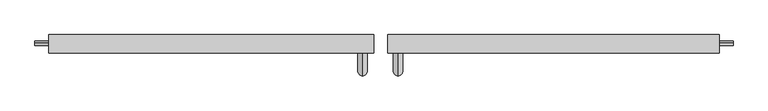
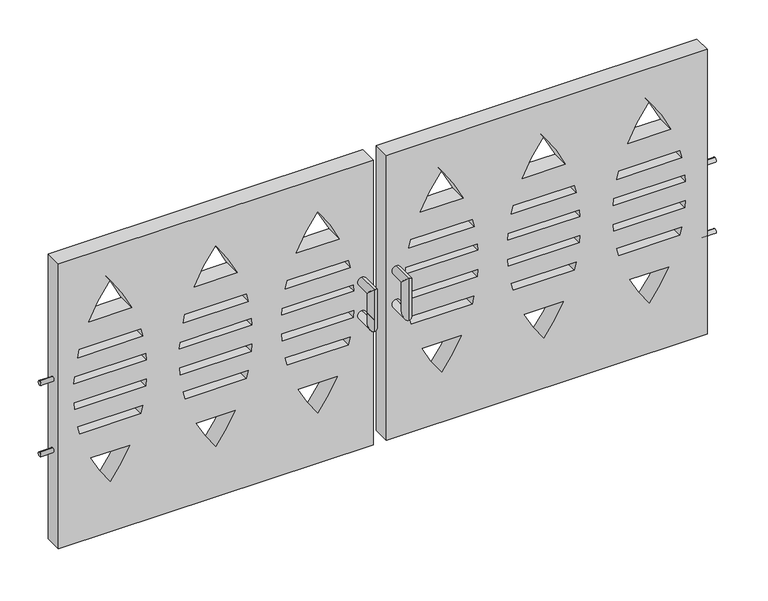
"""IFC4 building model written with IfcOpenShell, lengths in millimetres: proxy geometry."""

from ifc_helpers import new_model, si_unit, point, frame, frame_2d, origin, place, context, project, spatial, polyline, circle_curve, ellipse_curve, trimmed, segment, composite_curve, outline, extrude, source, transform, mapped, element, save
from ifc_brep_helpers import plane_surface, cylinder_surface, advanced_brep


def generic_models_af7f3ebe(model_context):
    return source(origin(), model_context, "Body", "SolidModel", [
        extrude(outline(polyline([(0.0, 268.7654616), (1727.2, 268.7654616), (1727.2, -1534.6345384), (0.0, -1534.6345384), (0.0, 268.7654616)]), holes=[composite_curve([segment(trimmed(circle_curve(frame_2d((913.3858921, 735.2120442)), 991.7835907), [point((1315.7032602, -171.3062546))], [point((1522.0610264, -47.8264425))], True, "CARTESIAN"), True, "CONTINUOUS"), segment(trimmed(circle_curve(frame_2d((913.3858921, -830.8649293)), 991.7835907), [point((1522.0610264, -47.8264425))], [point((1315.7032602, 75.6533695))], True, "CARTESIAN"), True, "CONTINUOUS"), segment(polyline([(1315.7032602, 75.6533695), (1315.7032602, -171.3062546)]), True, "CONTINUOUS")], self_intersect=False), composite_curve([segment(trimmed(circle_curve(frame_2d((913.3858921, -830.8649293)), 991.7835907), [point((1167.7706197, 127.7398387))], [point((1120.5108318, 139.0494742))], True, "CARTESIAN"), True, "CONTINUOUS"), segment(polyline([(1120.5108318, 139.0494742), (1120.5108318, -234.7023593)]), True, "CONTINUOUS"), segment(trimmed(circle_curve(frame_2d((913.3858921, 735.2120442)), 991.7835907), [point((1120.5108318, -234.7023593))], [point((1167.7706197, -223.3927238))], True, "CARTESIAN"), True, "CONTINUOUS"), segment(polyline([(1167.7706197, -223.3927238), (1167.7706197, 127.7398387)]), True, "CONTINUOUS")], self_intersect=False), composite_curve([segment(trimmed(circle_curve(frame_2d((913.3858921, -830.8649293)), 991.7835907), [point((1008.9376367, 156.3050434))], [point((969.7809206, 159.3139897))], True, "CARTESIAN"), True, "CONTINUOUS"), segment(polyline([(969.7809206, 159.3139897), (969.7809206, -254.9668748)]), True, "CONTINUOUS"), segment(trimmed(circle_curve(frame_2d((913.3858921, 735.2120442)), 991.7835907), [point((969.7809206, -254.9668748))], [point((1008.9376367, -251.9579284))], True, "CARTESIAN"), True, "CONTINUOUS"), segment(polyline([(1008.9376367, -251.9579284), (1008.9376367, 156.3050434)]), True, "CONTINUOUS")], self_intersect=False), composite_curve([segment(trimmed(circle_curve(frame_2d((913.3858921, -830.8649293)), 991.7835907), [point((853.4628105, 159.1067446))], [point((811.4921317, 155.6706009))], True, "CARTESIAN"), True, "CONTINUOUS"), segment(polyline([(811.4921317, 155.6706009), (811.4921317, -251.323486)]), True, "CONTINUOUS"), segment(trimmed(circle_curve(frame_2d((913.3858921, 735.2120442)), 991.7835907), [point((811.4921317, -251.323486))], [point((853.4628105, -254.7596297))], True, "CARTESIAN"), True, "CONTINUOUS"), segment(polyline([(853.4628105, -254.7596297), (853.4628105, 159.1067446)]), True, "CONTINUOUS")], self_intersect=False), composite_curve([segment(trimmed(circle_curve(frame_2d((913.3858921, -830.8649293)), 991.7835907), [point((700.6764218, 137.8400681))], [point((655.683383, 126.8532483))], True, "CARTESIAN"), True, "CONTINUOUS"), segment(polyline([(655.683383, 126.8532483), (655.683383, -222.5061333)]), True, "CONTINUOUS"), segment(trimmed(circle_curve(frame_2d((913.3858921, 735.2120442)), 991.7835907), [point((655.683383, -222.5061333))], [point((700.6764218, -233.4929532))], True, "CARTESIAN"), True, "CONTINUOUS"), segment(polyline([(700.6764218, -233.4929532), (700.6764218, 137.8400681)]), True, "CONTINUOUS")], self_intersect=False), composite_curve([segment(trimmed(circle_curve(frame_2d((913.3858921, -830.8649293)), 991.7835907), [point((485.5755246, 63.9048625))], [point((304.7107578, -47.8264425))], True, "CARTESIAN"), True, "CONTINUOUS"), segment(trimmed(circle_curve(frame_2d((913.3858921, 735.2120442)), 991.7835907), [point((304.7107578, -47.8264425))], [point((485.5755246, -159.5577476))], True, "CARTESIAN"), True, "CONTINUOUS"), segment(polyline([(485.5755246, -159.5577476), (485.5755246, 63.9048625)]), True, "CONTINUOUS")], self_intersect=False), composite_curve([segment(polyline([(1315.7032602, -510.0774949), (1315.7032602, -757.0371191)]), True, "CONTINUOUS"), segment(trimmed(circle_curve(frame_2d((913.3858921, 149.4811798)), 991.7835907), [point((1315.7032602, -757.0371191))], [point((1522.0610264, -633.557307))], True, "CARTESIAN"), True, "CONTINUOUS"), segment(trimmed(circle_curve(frame_2d((913.3858921, -1416.5957937)), 991.7835907), [point((1522.0610264, -633.557307))], [point((1315.7032602, -510.0774949))], True, "CARTESIAN"), True, "CONTINUOUS")], self_intersect=False), composite_curve([segment(polyline([(1167.7706197, -809.1235882), (1167.7706197, -457.9910257)]), True, "CONTINUOUS"), segment(trimmed(circle_curve(frame_2d((913.3858921, -1416.5957937)), 991.7835907), [point((1167.7706197, -457.9910257))], [point((1120.5108318, -446.6813902))], True, "CARTESIAN"), True, "CONTINUOUS"), segment(polyline([(1120.5108318, -446.6813902), (1120.5108318, -820.4332237)]), True, "CONTINUOUS"), segment(trimmed(circle_curve(frame_2d((913.3858921, 149.4811798)), 991.7835907), [point((1120.5108318, -820.4332237))], [point((1167.7706197, -809.1235882))], True, "CARTESIAN"), True, "CONTINUOUS")], self_intersect=False), composite_curve([segment(polyline([(1008.9376367, -837.6887929), (1008.9376367, -429.4258211)]), True, "CONTINUOUS"), segment(trimmed(circle_curve(frame_2d((913.3858921, -1416.5957937)), 991.7835907), [point((1008.9376367, -429.4258211))], [point((969.7809206, -426.4168748))], True, "CARTESIAN"), True, "CONTINUOUS"), segment(polyline([(969.7809206, -426.4168748), (969.7809206, -840.6977392)]), True, "CONTINUOUS"), segment(trimmed(circle_curve(frame_2d((913.3858921, 149.4811798)), 991.7835907), [point((969.7809206, -840.6977392))], [point((1008.9376367, -837.6887929))], True, "CARTESIAN"), True, "CONTINUOUS")], self_intersect=False), composite_curve([segment(polyline([(853.4628105, -840.4904941), (853.4628105, -426.6241198)]), True, "CONTINUOUS"), segment(trimmed(circle_curve(frame_2d((913.3858921, -1416.5957937)), 991.7835907), [point((853.4628105, -426.6241198))], [point((811.4921317, -430.0602635))], True, "CARTESIAN"), True, "CONTINUOUS"), segment(polyline([(811.4921317, -430.0602635), (811.4921317, -837.0543504)]), True, "CONTINUOUS"), segment(trimmed(circle_curve(frame_2d((913.3858921, 149.4811798)), 991.7835907), [point((811.4921317, -837.0543504))], [point((853.4628105, -840.4904941))], True, "CARTESIAN"), True, "CONTINUOUS")], self_intersect=False), composite_curve([segment(polyline([(700.6764218, -819.2238176), (700.6764218, -447.8907963)]), True, "CONTINUOUS"), segment(trimmed(circle_curve(frame_2d((913.3858921, -1416.5957937)), 991.7835907), [point((700.6764218, -447.8907963))], [point((655.683383, -458.8776162))], True, "CARTESIAN"), True, "CONTINUOUS"), segment(polyline([(655.683383, -458.8776162), (655.683383, -808.2369978)]), True, "CONTINUOUS"), segment(trimmed(circle_curve(frame_2d((913.3858921, 149.4811798)), 991.7835907), [point((655.683383, -808.2369978))], [point((700.6764218, -819.2238176))], True, "CARTESIAN"), True, "CONTINUOUS")], self_intersect=False), composite_curve([segment(polyline([(485.5755246, -745.288612), (485.5755246, -521.8260019)]), True, "CONTINUOUS"), segment(trimmed(circle_curve(frame_2d((913.3858921, -1416.5957937)), 991.7835907), [point((485.5755246, -521.8260019))], [point((304.7107578, -633.557307))], True, "CARTESIAN"), True, "CONTINUOUS"), segment(trimmed(circle_curve(frame_2d((913.3858921, 149.4811798)), 991.7835907), [point((304.7107578, -633.557307))], [point((485.5755246, -745.288612))], True, "CARTESIAN"), True, "CONTINUOUS")], self_intersect=False), composite_curve([segment(trimmed(circle_curve(frame_2d((913.3858921, -455.2996847)), 991.7835907), [point((1315.7032602, -1361.8179835))], [point((1522.0610264, -1238.3381714))], True, "CARTESIAN"), True, "CONTINUOUS"), segment(trimmed(circle_curve(frame_2d((913.3858921, -2021.3766581)), 991.7835907), [point((1522.0610264, -1238.3381714))], [point((1315.7032602, -1114.8583593))], True, "CARTESIAN"), True, "CONTINUOUS"), segment(polyline([(1315.7032602, -1114.8583593), (1315.7032602, -1361.8179835)]), True, "CONTINUOUS")], self_intersect=False), composite_curve([segment(trimmed(circle_curve(frame_2d((913.3858921, -2021.3766581)), 991.7835907), [point((1167.7706197, -1062.7718902))], [point((1120.5108318, -1051.4622546))], True, "CARTESIAN"), True, "CONTINUOUS"), segment(polyline([(1120.5108318, -1051.4622546), (1120.5108318, -1425.2140882)]), True, "CONTINUOUS"), segment(trimmed(circle_curve(frame_2d((913.3858921, -455.2996847)), 991.7835907), [point((1120.5108318, -1425.2140882))], [point((1167.7706197, -1413.9044526))], True, "CARTESIAN"), True, "CONTINUOUS"), segment(polyline([(1167.7706197, -1413.9044526), (1167.7706197, -1062.7718902)]), True, "CONTINUOUS")], self_intersect=False), composite_curve([segment(trimmed(circle_curve(frame_2d((913.3858921, -2021.3766581)), 991.7835907), [point((1008.9376367, -1034.2066855))], [point((969.7809206, -1031.1977392))], True, "CARTESIAN"), True, "CONTINUOUS"), segment(polyline([(969.7809206, -1031.1977392), (969.7809206, -1445.4786036)]), True, "CONTINUOUS"), segment(trimmed(circle_curve(frame_2d((913.3858921, -455.2996847)), 991.7835907), [point((969.7809206, -1445.4786036))], [point((1008.9376367, -1442.4696573))], True, "CARTESIAN"), True, "CONTINUOUS"), segment(polyline([(1008.9376367, -1442.4696573), (1008.9376367, -1034.2066855)]), True, "CONTINUOUS")], self_intersect=False), composite_curve([segment(trimmed(circle_curve(frame_2d((913.3858921, -2021.3766581)), 991.7835907), [point((853.4628105, -1031.4049843))], [point((811.4921317, -1034.8411279))], True, "CARTESIAN"), True, "CONTINUOUS"), segment(polyline([(811.4921317, -1034.8411279), (811.4921317, -1441.8352149)]), True, "CONTINUOUS"), segment(trimmed(circle_curve(frame_2d((913.3858921, -455.2996847)), 991.7835907), [point((811.4921317, -1441.8352149))], [point((853.4628105, -1445.2713585))], True, "CARTESIAN"), True, "CONTINUOUS"), segment(polyline([(853.4628105, -1445.2713585), (853.4628105, -1031.4049843)]), True, "CONTINUOUS")], self_intersect=False), composite_curve([segment(trimmed(circle_curve(frame_2d((913.3858921, -2021.3766581)), 991.7835907), [point((700.6764218, -1052.6716607))], [point((655.683383, -1063.6584806))], True, "CARTESIAN"), True, "CONTINUOUS"), segment(polyline([(655.683383, -1063.6584806), (655.683383, -1413.0178622)]), True, "CONTINUOUS"), segment(trimmed(circle_curve(frame_2d((913.3858921, -455.2996847)), 991.7835907), [point((655.683383, -1413.0178622))], [point((700.6764218, -1424.0046821))], True, "CARTESIAN"), True, "CONTINUOUS"), segment(polyline([(700.6764218, -1424.0046821), (700.6764218, -1052.6716607)]), True, "CONTINUOUS")], self_intersect=False), composite_curve([segment(trimmed(circle_curve(frame_2d((913.3858921, -2021.3766581)), 991.7835907), [point((485.5755246, -1126.6068664))], [point((304.7107578, -1238.3381714))], True, "CARTESIAN"), True, "CONTINUOUS"), segment(trimmed(circle_curve(frame_2d((913.3858921, -455.2996847)), 991.7835907), [point((304.7107578, -1238.3381714))], [point((485.5755246, -1350.0694764))], True, "CARTESIAN"), True, "CONTINUOUS"), segment(polyline([(485.5755246, -1350.0694764), (485.5755246, -1126.6068664)]), True, "CONTINUOUS")], self_intersect=False)]), frame((0.0, -101.6, 0.0), z_axis=(0.0, 1.0, 0.0), x_axis=(0.0, 0.0, 1.0)), (0.0, 0.0, 1.0), 101.6),
        extrude(outline(polyline([(1727.2, 2183.266195), (1727.2, 344.9654616), (0.0, 344.9654616), (0.0, 2183.266195), (1727.2, 2183.266195)]), holes=[composite_curve([segment(polyline([(1315.7032602, 785.0371778), (1315.7032602, 538.0775536)]), True, "CONTINUOUS"), segment(trimmed(circle_curve(frame_2d((913.3858921, 1444.5958525)), 991.7835907), [point((1315.7032602, 538.0775536))], [point((1522.0610264, 661.5573657))], True, "CARTESIAN"), True, "CONTINUOUS"), segment(trimmed(circle_curve(frame_2d((913.3858921, -121.481121)), 991.7835907), [point((1522.0610264, 661.5573657))], [point((1315.7032602, 785.0371778))], True, "CARTESIAN"), True, "CONTINUOUS")], self_intersect=False), composite_curve([segment(polyline([(1167.7706197, 485.9910845), (1167.7706197, 837.1236469)]), True, "CONTINUOUS"), segment(trimmed(circle_curve(frame_2d((913.3858921, -121.481121)), 991.7835907), [point((1167.7706197, 837.1236469))], [point((1120.5108318, 848.4332825))], True, "CARTESIAN"), True, "CONTINUOUS"), segment(polyline([(1120.5108318, 848.4332825), (1120.5108318, 474.681449)]), True, "CONTINUOUS"), segment(trimmed(circle_curve(frame_2d((913.3858921, 1444.5958525)), 991.7835907), [point((1120.5108318, 474.681449))], [point((1167.7706197, 485.9910845))], True, "CARTESIAN"), True, "CONTINUOUS")], self_intersect=False), composite_curve([segment(polyline([(1008.9376367, 457.4258798), (1008.9376367, 865.6888516)]), True, "CONTINUOUS"), segment(trimmed(circle_curve(frame_2d((913.3858921, -121.481121)), 991.7835907), [point((1008.9376367, 865.6888516))], [point((969.7809206, 868.6977979))], True, "CARTESIAN"), True, "CONTINUOUS"), segment(polyline([(969.7809206, 868.6977979), (969.7809206, 454.4169335)]), True, "CONTINUOUS"), segment(trimmed(circle_curve(frame_2d((913.3858921, 1444.5958525)), 991.7835907), [point((969.7809206, 454.4169335))], [point((1008.9376367, 457.4258798))], True, "CARTESIAN"), True, "CONTINUOUS")], self_intersect=False), composite_curve([segment(polyline([(853.4628105, 454.6241786), (853.4628105, 868.4905529)]), True, "CONTINUOUS"), segment(trimmed(circle_curve(frame_2d((913.3858921, -121.481121)), 991.7835907), [point((853.4628105, 868.4905529))], [point((811.4921317, 865.0544092))], True, "CARTESIAN"), True, "CONTINUOUS"), segment(polyline([(811.4921317, 865.0544092), (811.4921317, 458.0603222)]), True, "CONTINUOUS"), segment(trimmed(circle_curve(frame_2d((913.3858921, 1444.5958525)), 991.7835907), [point((811.4921317, 458.0603222))], [point((853.4628105, 454.6241786))], True, "CARTESIAN"), True, "CONTINUOUS")], self_intersect=False), composite_curve([segment(polyline([(700.6764218, 475.890855), (700.6764218, 847.2238764)]), True, "CONTINUOUS"), segment(trimmed(circle_curve(frame_2d((913.3858921, -121.481121)), 991.7835907), [point((700.6764218, 847.2238764))], [point((655.683383, 836.2370565))], True, "CARTESIAN"), True, "CONTINUOUS"), segment(polyline([(655.683383, 836.2370565), (655.683383, 486.8776749)]), True, "CONTINUOUS"), segment(trimmed(circle_curve(frame_2d((913.3858921, 1444.5958525)), 991.7835907), [point((655.683383, 486.8776749))], [point((700.6764218, 475.890855))], True, "CARTESIAN"), True, "CONTINUOUS")], self_intersect=False), composite_curve([segment(polyline([(485.5755246, 549.8260607), (485.5755246, 773.2886707)]), True, "CONTINUOUS"), segment(trimmed(circle_curve(frame_2d((913.3858921, -121.481121)), 991.7835907), [point((485.5755246, 773.2886707))], [point((304.7107578, 661.5573657))], True, "CARTESIAN"), True, "CONTINUOUS"), segment(trimmed(circle_curve(frame_2d((913.3858921, 1444.5958525)), 991.7835907), [point((304.7107578, 661.5573657))], [point((485.5755246, 549.8260607))], True, "CARTESIAN"), True, "CONTINUOUS")], self_intersect=False), composite_curve([segment(trimmed(circle_curve(frame_2d((913.3858921, 2030.3267169)), 991.7835907), [point((1315.7032602, 1123.8084181))], [point((1522.0610264, 1247.2882301))], True, "CARTESIAN"), True, "CONTINUOUS"), segment(trimmed(circle_curve(frame_2d((913.3858921, 464.2497434)), 991.7835907), [point((1522.0610264, 1247.2882301))], [point((1315.7032602, 1370.7680422))], True, "CARTESIAN"), True, "CONTINUOUS"), segment(polyline([(1315.7032602, 1370.7680422), (1315.7032602, 1123.8084181)]), True, "CONTINUOUS")], self_intersect=False), composite_curve([segment(trimmed(circle_curve(frame_2d((913.3858921, 464.2497434)), 991.7835907), [point((1167.7706197, 1422.8545114))], [point((1120.5108318, 1434.1641469))], True, "CARTESIAN"), True, "CONTINUOUS"), segment(polyline([(1120.5108318, 1434.1641469), (1120.5108318, 1060.4123134)]), True, "CONTINUOUS"), segment(trimmed(circle_curve(frame_2d((913.3858921, 2030.3267169)), 991.7835907), [point((1120.5108318, 1060.4123134))], [point((1167.7706197, 1071.7219489))], True, "CARTESIAN"), True, "CONTINUOUS"), segment(polyline([(1167.7706197, 1071.7219489), (1167.7706197, 1422.8545114)]), True, "CONTINUOUS")], self_intersect=False), composite_curve([segment(trimmed(circle_curve(frame_2d((913.3858921, 464.2497434)), 991.7835907), [point((1008.9376367, 1451.419716))], [point((969.7809206, 1454.4286624))], True, "CARTESIAN"), True, "CONTINUOUS"), segment(polyline([(969.7809206, 1454.4286624), (969.7809206, 1040.1477979)]), True, "CONTINUOUS"), segment(trimmed(circle_curve(frame_2d((913.3858921, 2030.3267169)), 991.7835907), [point((969.7809206, 1040.1477979))], [point((1008.9376367, 1043.1567442))], True, "CARTESIAN"), True, "CONTINUOUS"), segment(polyline([(1008.9376367, 1043.1567442), (1008.9376367, 1451.419716)]), True, "CONTINUOUS")], self_intersect=False), composite_curve([segment(trimmed(circle_curve(frame_2d((913.3858921, 464.2497434)), 991.7835907), [point((853.4628105, 1454.2214173))], [point((811.4921317, 1450.7852736))], True, "CARTESIAN"), True, "CONTINUOUS"), segment(polyline([(811.4921317, 1450.7852736), (811.4921317, 1043.7911867)]), True, "CONTINUOUS"), segment(trimmed(circle_curve(frame_2d((913.3858921, 2030.3267169)), 991.7835907), [point((811.4921317, 1043.7911867))], [point((853.4628105, 1040.355043))], True, "CARTESIAN"), True, "CONTINUOUS"), segment(polyline([(853.4628105, 1040.355043), (853.4628105, 1454.2214173)]), True, "CONTINUOUS")], self_intersect=False), composite_curve([segment(trimmed(circle_curve(frame_2d((913.3858921, 464.2497434)), 991.7835907), [point((700.6764218, 1432.9547408))], [point((655.683383, 1421.9679209))], True, "CARTESIAN"), True, "CONTINUOUS"), segment(polyline([(655.683383, 1421.9679209), (655.683383, 1072.6085394)]), True, "CONTINUOUS"), segment(trimmed(circle_curve(frame_2d((913.3858921, 2030.3267169)), 991.7835907), [point((655.683383, 1072.6085394))], [point((700.6764218, 1061.6217195))], True, "CARTESIAN"), True, "CONTINUOUS"), segment(polyline([(700.6764218, 1061.6217195), (700.6764218, 1432.9547408)]), True, "CONTINUOUS")], self_intersect=False), composite_curve([segment(trimmed(circle_curve(frame_2d((913.3858921, 464.2497434)), 991.7835907), [point((485.5755246, 1359.0195352))], [point((304.7107578, 1247.2882301))], True, "CARTESIAN"), True, "CONTINUOUS"), segment(trimmed(circle_curve(frame_2d((913.3858921, 2030.3267169)), 991.7835907), [point((304.7107578, 1247.2882301))], [point((485.5755246, 1135.5569251))], True, "CARTESIAN"), True, "CONTINUOUS"), segment(polyline([(485.5755246, 1135.5569251), (485.5755246, 1359.0195352)]), True, "CONTINUOUS")], self_intersect=False), composite_curve([segment(polyline([(1315.7032602, 1975.5489067), (1315.7032602, 1728.5892825)]), True, "CONTINUOUS"), segment(trimmed(circle_curve(frame_2d((913.3858921, 2635.1075813)), 991.7835907), [point((1315.7032602, 1728.5892825))], [point((1522.0610264, 1852.0690946))], True, "CARTESIAN"), True, "CONTINUOUS"), segment(trimmed(circle_curve(frame_2d((913.3858921, 1069.0306078)), 991.7835907), [point((1522.0610264, 1852.0690946))], [point((1315.7032602, 1975.5489067))], True, "CARTESIAN"), True, "CONTINUOUS")], self_intersect=False), composite_curve([segment(polyline([(1167.7706197, 1676.5028134), (1167.7706197, 2027.6353758)]), True, "CONTINUOUS"), segment(trimmed(circle_curve(frame_2d((913.3858921, 1069.0306078)), 991.7835907), [point((1167.7706197, 2027.6353758))], [point((1120.5108318, 2038.9450113))], True, "CARTESIAN"), True, "CONTINUOUS"), segment(polyline([(1120.5108318, 2038.9450113), (1120.5108318, 1665.1931778)]), True, "CONTINUOUS"), segment(trimmed(circle_curve(frame_2d((913.3858921, 2635.1075813)), 991.7835907), [point((1120.5108318, 1665.1931778))], [point((1167.7706197, 1676.5028134))], True, "CARTESIAN"), True, "CONTINUOUS")], self_intersect=False), composite_curve([segment(polyline([(1008.9376367, 1647.9376087), (1008.9376367, 2056.2005805)]), True, "CONTINUOUS"), segment(trimmed(circle_curve(frame_2d((913.3858921, 1069.0306078)), 991.7835907), [point((1008.9376367, 2056.2005805))], [point((969.7809206, 2059.2095268))], True, "CARTESIAN"), True, "CONTINUOUS"), segment(polyline([(969.7809206, 2059.2095268), (969.7809206, 1644.9286624)]), True, "CONTINUOUS"), segment(trimmed(circle_curve(frame_2d((913.3858921, 2635.1075813)), 991.7835907), [point((969.7809206, 1644.9286624))], [point((1008.9376367, 1647.9376087))], True, "CARTESIAN"), True, "CONTINUOUS")], self_intersect=False), composite_curve([segment(polyline([(853.4628105, 1645.1359074), (853.4628105, 2059.0022817)]), True, "CONTINUOUS"), segment(trimmed(circle_curve(frame_2d((913.3858921, 1069.0306078)), 991.7835907), [point((853.4628105, 2059.0022817))], [point((811.4921317, 2055.566138))], True, "CARTESIAN"), True, "CONTINUOUS"), segment(polyline([(811.4921317, 2055.566138), (811.4921317, 1648.5720511)]), True, "CONTINUOUS"), segment(trimmed(circle_curve(frame_2d((913.3858921, 2635.1075813)), 991.7835907), [point((811.4921317, 1648.5720511))], [point((853.4628105, 1645.1359074))], True, "CARTESIAN"), True, "CONTINUOUS")], self_intersect=False), composite_curve([segment(polyline([(700.6764218, 1666.4025839), (700.6764218, 2037.7356052)]), True, "CONTINUOUS"), segment(trimmed(circle_curve(frame_2d((913.3858921, 1069.0306078)), 991.7835907), [point((700.6764218, 2037.7356052))], [point((655.683383, 2026.7487854))], True, "CARTESIAN"), True, "CONTINUOUS"), segment(polyline([(655.683383, 2026.7487854), (655.683383, 1677.3894038)]), True, "CONTINUOUS"), segment(trimmed(circle_curve(frame_2d((913.3858921, 2635.1075813)), 991.7835907), [point((655.683383, 1677.3894038))], [point((700.6764218, 1666.4025839))], True, "CARTESIAN"), True, "CONTINUOUS")], self_intersect=False), composite_curve([segment(polyline([(485.5755246, 1740.3377895), (485.5755246, 1963.8003996)]), True, "CONTINUOUS"), segment(trimmed(circle_curve(frame_2d((913.3858921, 1069.0306078)), 991.7835907), [point((485.5755246, 1963.8003996))], [point((304.7107578, 1852.0690946))], True, "CARTESIAN"), True, "CONTINUOUS"), segment(trimmed(circle_curve(frame_2d((913.3858921, 2635.1075813)), 991.7835907), [point((304.7107578, 1852.0690946))], [point((485.5755246, 1740.3377895))], True, "CARTESIAN"), True, "CONTINUOUS")], self_intersect=False)]), frame((0.0, -101.6, 0.0), z_axis=(0.0, 1.0, 0.0), x_axis=(0.0, 0.0, 1.0)), (0.0, 0.0, 1.0), 101.6),
        advanced_brep(
        [(205.2654616, -101.6, 1039.4610264), (205.2654616, -101.6, 988.6610264), (205.2654616, -101.6, 785.4610264), (205.2654616, -101.6, 836.2610264), (205.2654616, -228.6, 1039.4610264), (205.2654616, -177.8, 988.6610264), (205.2654616, -228.6, 785.4610264), (205.2654616, -177.8, 836.2610264)],
        [
            (0, 1, circle_curve(frame((205.2654616, -101.6, 1014.0610264), z_axis=(0.0, 1.0, 0.0), x_axis=(0.0, 0.0, -1.0)), 25.4)),
            (1, 0, circle_curve(frame((205.2654616, -101.6, 1014.0610264), z_axis=(0.0, 1.0, 0.0), x_axis=(0.0, 0.0, -1.0)), 25.4)),
            (2, 3, circle_curve(frame((205.2654616, -101.6, 810.8610264), z_axis=(0.0, 1.0, 0.0), x_axis=(0.0, 0.0, 1.0)), 25.4)),
            (3, 2, circle_curve(frame((205.2654616, -101.6, 810.8610264), z_axis=(0.0, 1.0, 0.0), x_axis=(0.0, 0.0, 1.0)), 25.4)),
            (0, 4),
            (4, 5, ellipse_curve(frame((205.2654616, -203.2, 1014.0610264), z_axis=(0.0, 0.7071067811865495, 0.7071067811865455), x_axis=(0.0, 0.7071067811865457, -0.7071067811865493)), 35.9210245, 25.4)),
            (5, 1),
            (5, 4, ellipse_curve(frame((205.2654616, -203.2, 1014.0610264), z_axis=(0.0, 0.7071067811865495, 0.7071067811865455), x_axis=(0.0, 0.7071067811865457, -0.7071067811865493)), 35.9210245, 25.4)),
            (4, 6),
            (6, 7, ellipse_curve(frame((205.2654616, -203.2, 810.8610264), z_axis=(0.0, -0.7071067811865457, 0.7071067811865495), x_axis=(0.0, 0.7071067811865496, 0.7071067811865455)), 35.9210245, 25.4)),
            (7, 5),
            (7, 6, ellipse_curve(frame((205.2654616, -203.2, 810.8610264), z_axis=(0.0, -0.7071067811865457, 0.7071067811865495), x_axis=(0.0, 0.7071067811865496, 0.7071067811865455)), 35.9210245, 25.4)),
            (6, 2),
            (3, 7),
        ],
        [
            plane_surface(frame((205.2654616, -101.6, 1014.0610264), z_axis=(0.0, 1.0, 0.0), x_axis=(1.0, 0.0, 0.0))),
            plane_surface(frame((205.2654616, -101.6, 810.8610264), z_axis=(0.0, 1.0, 0.0), x_axis=(1.0, 0.0, 0.0))),
            cylinder_surface(frame((205.2654616, -101.6, 1014.0610264), z_axis=(0.0, 1.0, 0.0), x_axis=(0.0, 0.0, -1.0)), 25.4),
            cylinder_surface(frame((205.2654616, -203.2, 1014.0610264), z_axis=(0.0, 0.0, 1.0), x_axis=(0.0, 1.0, 0.0)), 25.4),
            cylinder_surface(frame((205.2654616, -203.2, 810.8610264), z_axis=(0.0, -1.0, 0.0), x_axis=(0.0, 0.0, 1.0)), 25.4),
        ],
        [
            (0, [[1, 2]]),
            (1, [[3, 4]]),
            (2, [[-1, 5, 6, 7]]),
            (2, [[-2, -7, 8, -5]]),
            (3, [[-6, 9, 10, 11]]),
            (3, [[-8, -11, 12, -9]]),
            (4, [[-10, 13, -4, 14]]),
            (4, [[-12, -14, -3, -13]]),
        ],
    ),
        advanced_brep(
        [(402.1154616, -101.6, 1039.4610264), (402.1154616, -101.6, 988.6610264), (402.1154616, -101.6, 785.4610264), (402.1154616, -101.6, 836.2610264), (402.1154616, -228.6, 1039.4610264), (402.1154616, -177.8, 988.6610264), (402.1154616, -228.6, 785.4610264), (402.1154616, -177.8, 836.2610264)],
        [
            (0, 1, circle_curve(frame((402.1154616, -101.6, 1014.0610264), z_axis=(0.0, 1.0, 0.0), x_axis=(0.0, 0.0, -1.0)), 25.4)),
            (1, 0, circle_curve(frame((402.1154616, -101.6, 1014.0610264), z_axis=(0.0, 1.0, 0.0), x_axis=(0.0, 0.0, -1.0)), 25.4)),
            (2, 3, circle_curve(frame((402.1154616, -101.6, 810.8610264), z_axis=(0.0, 1.0, 0.0), x_axis=(0.0, 0.0, 1.0)), 25.4)),
            (3, 2, circle_curve(frame((402.1154616, -101.6, 810.8610264), z_axis=(0.0, 1.0, 0.0), x_axis=(0.0, 0.0, 1.0)), 25.4)),
            (0, 4),
            (4, 5, ellipse_curve(frame((402.1154616, -203.2, 1014.0610264), z_axis=(0.0, 0.7071067811865495, 0.7071067811865455), x_axis=(0.0, 0.7071067811865457, -0.7071067811865493)), 35.9210245, 25.4)),
            (5, 1),
            (5, 4, ellipse_curve(frame((402.1154616, -203.2, 1014.0610264), z_axis=(0.0, 0.7071067811865495, 0.7071067811865455), x_axis=(0.0, 0.7071067811865457, -0.7071067811865493)), 35.9210245, 25.4)),
            (4, 6),
            (6, 7, ellipse_curve(frame((402.1154616, -203.2, 810.8610264), z_axis=(0.0, -0.7071067811865457, 0.7071067811865495), x_axis=(0.0, 0.7071067811865496, 0.7071067811865455)), 35.9210245, 25.4)),
            (7, 5),
            (7, 6, ellipse_curve(frame((402.1154616, -203.2, 810.8610264), z_axis=(0.0, -0.7071067811865457, 0.7071067811865495), x_axis=(0.0, 0.7071067811865496, 0.7071067811865455)), 35.9210245, 25.4)),
            (6, 2),
            (3, 7),
        ],
        [
            plane_surface(frame((402.1154616, -101.6, 1014.0610264), z_axis=(0.0, 1.0, 0.0), x_axis=(1.0, 0.0, 0.0))),
            plane_surface(frame((402.1154616, -101.6, 810.8610264), z_axis=(0.0, 1.0, 0.0), x_axis=(1.0, 0.0, 0.0))),
            cylinder_surface(frame((402.1154616, -101.6, 1014.0610264), z_axis=(0.0, 1.0, 0.0), x_axis=(0.0, 0.0, -1.0)), 25.4),
            cylinder_surface(frame((402.1154616, -203.2, 1014.0610264), z_axis=(0.0, 0.0, 1.0), x_axis=(0.0, 1.0, 0.0)), 25.4),
            cylinder_surface(frame((402.1154616, -203.2, 810.8610264), z_axis=(0.0, -1.0, 0.0), x_axis=(0.0, 0.0, 1.0)), 25.4),
        ],
        [
            (0, [[1, 2]]),
            (1, [[3, 4]]),
            (2, [[-1, 5, 6, 7]]),
            (2, [[-2, -7, 8, -5]]),
            (3, [[-6, 9, 10, 11]]),
            (3, [[-8, -11, 12, -9]]),
            (4, [[-10, 13, -4, 14]]),
            (4, [[-12, -14, -3, -13]]),
        ],
    ),
        extrude(outline(composite_curve([segment(trimmed(circle_curve(frame_2d((-47.1865605, 998.9501685)), 12.7), [point((-47.1865605, 1011.6501685))], [point((-47.1865605, 986.2501685))], False, "CARTESIAN"), True, "CONTINUOUS"), segment(trimmed(circle_curve(frame_2d((-47.1865605, 998.9501685)), 12.7), [point((-47.1865605, 986.2501685))], [point((-47.1865605, 1011.6501685))], False, "CARTESIAN"), True, "CONTINUOUS")], self_intersect=False)), frame((2183.266195, 0.0, 0.0), z_axis=(1.0, 0.0, 0.0), x_axis=(0.0, 1.0, 0.0)), (0.0, 0.0, 1.0), 76.2),
        extrude(outline(composite_curve([segment(trimmed(circle_curve(frame_2d((-47.1865605, 567.1501685)), 12.7), [point((-47.1865605, 579.8501685))], [point((-47.1865605, 554.4501685))], False, "CARTESIAN"), True, "CONTINUOUS"), segment(trimmed(circle_curve(frame_2d((-47.1865605, 567.1501685)), 12.7), [point((-47.1865605, 554.4501685))], [point((-47.1865605, 579.8501685))], False, "CARTESIAN"), True, "CONTINUOUS")], self_intersect=False)), frame((2183.266195, 0.0, 0.0), z_axis=(1.0, 0.0, 0.0), x_axis=(0.0, 1.0, 0.0)), (0.0, 0.0, 1.0), 76.2),
        extrude(outline(composite_curve([segment(trimmed(circle_curve(frame_2d((-47.1865605, 998.9501685)), 12.7), [point((-47.1865605, 1011.6501685))], [point((-47.1865605, 986.2501685))], False, "CARTESIAN"), True, "CONTINUOUS"), segment(trimmed(circle_curve(frame_2d((-47.1865605, 998.9501685)), 12.7), [point((-47.1865605, 986.2501685))], [point((-47.1865605, 1011.6501685))], False, "CARTESIAN"), True, "CONTINUOUS")], self_intersect=False)), frame((-1610.8345384, 0.0, 0.0), z_axis=(1.0, 0.0, 0.0), x_axis=(0.0, 1.0, 0.0)), (0.0, 0.0, 1.0), 76.2),
        extrude(outline(composite_curve([segment(trimmed(circle_curve(frame_2d((-47.1865605, 567.1501685)), 12.7), [point((-47.1865605, 579.8501685))], [point((-47.1865605, 554.4501685))], False, "CARTESIAN"), True, "CONTINUOUS"), segment(trimmed(circle_curve(frame_2d((-47.1865605, 567.1501685)), 12.7), [point((-47.1865605, 554.4501685))], [point((-47.1865605, 579.8501685))], False, "CARTESIAN"), True, "CONTINUOUS")], self_intersect=False)), frame((-1610.8345384, 0.0, 0.0), z_axis=(1.0, 0.0, 0.0), x_axis=(0.0, 1.0, 0.0)), (0.0, 0.0, 1.0), 76.2),
    ])


if __name__ == "__main__":
    model = new_model("IFC4")
    model_context = context("Model", 3, world=origin())
    ifc_project = project(units=[si_unit("LENGTHUNIT", "METRE", prefix="MILLI")], contexts=[model_context])
    site = spatial("IfcSite", under=ifc_project)
    building = spatial("IfcBuilding", under=site)
    placement = place(None, origin())
    generic_models_shape = generic_models_af7f3ebe(model_context)
    element("IfcBuildingElementProxy", 1, Name="Generic Models", at=placement, inside=building, context=model_context, shape_type="MappedRepresentation", body=[
        mapped(generic_models_shape, transform((0.0, 0.0, 0.0), x_axis=(1.0, 0.0, 0.0), y_axis=(0.0, 1.0, 0.0), z_axis=(0.0, 0.0, 1.0))),
    ])
    save(model, "model.ifc")

# Revit data of these elements
# Type
#   Default Elevation = 0
# Element 1 (IfcBuildingElementProxy)
#   Materials on its faces: "GATE"
# Materials
#   "GATE": class "Generic", colour RGB 120 120 120, transparency 0, Cost = 0
